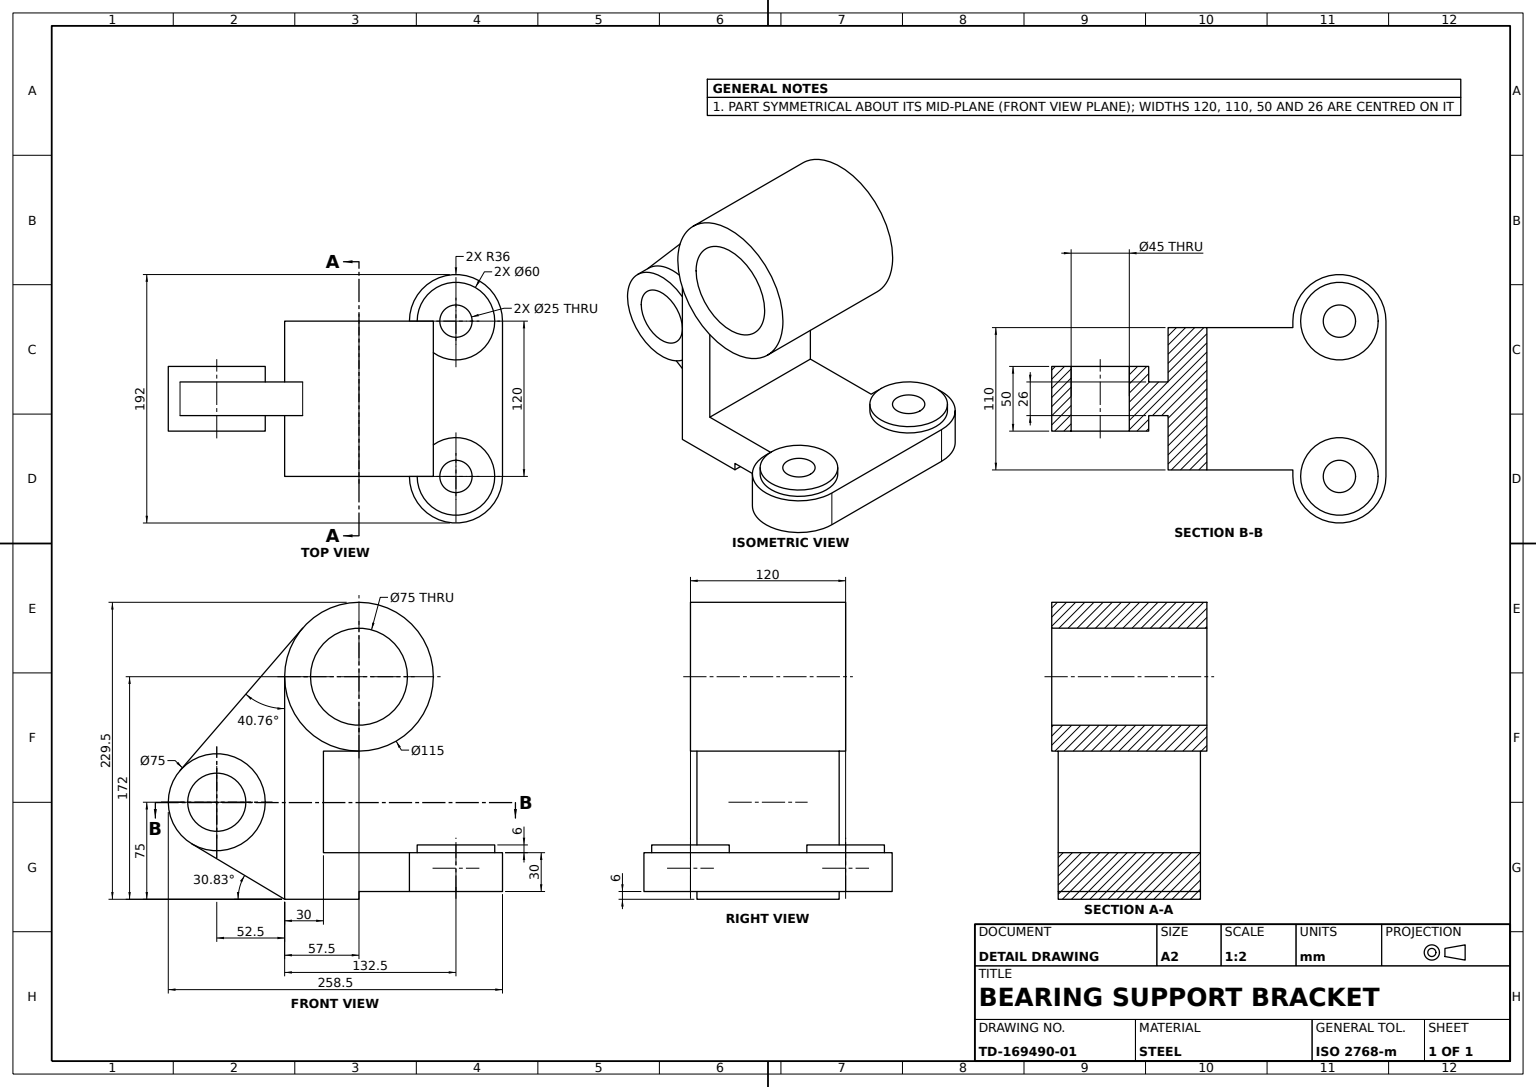
SolidWorks part; units mm, degrees
material "Plain Carbon Steel"
ref_plane "Front Plane" through (0, 0, 0) normal (0, 0, 1) x (1, 0, 0)
ref_plane "Top Plane" through (0, 0, 0) normal (0, 1, 0) x (1, 0, 0)
ref_plane "Right Plane" through (0, 0, 0) normal (1, 0, 0) x (0, 0, -1)
sketch "Bearing Housing Sketch" plane through (0, 0, 0) normal (1, 0, 0) x (0, 0, -1)
  circle A0 centre (0, 0) radius 37.5
  circle A1 centre (0, 0) radius 57.5
  dimension "D1" = 115
  dimension "D2" = 75
extrude "Bearing Housing Ø115" add sketch "Bearing Housing Sketch" against normal mid plane 120
ref_plane "Plane1" through (0, -166, 0) normal (0, 1, 0) x (1, 0, 0)
sketch "Base Foot Sketch" plane through (0, -166, 0) normal (0, 1, 0) x (1, 0, 0)
  line L0 (-60, 75) -> (60, 75) construction
  line L1 (-60, 111) -> (60, 111)
  line L2 (-60, 39) -> (60, 39)
  line L3 (-60, -57.5) -> (60, -57.5) construction
  arc A0 (-60, 111) -> (-60, 39) centre (-60, 75) ccw
  arc A1 (60, 39) -> (60, 111) centre (60, 75) ccw
  circle A2 centre (60, 75) radius 12.5
  circle A3 centre (-60, 75) radius 12.5
  point P2 (0, 75)
  dimension "D2" = 36
  dimension "D4" = 25
  dimension "D5" = 25
  dimension "D1" = 120
  dimension "D3" = 132.5
extrude "Base Foot" add sketch "Base Foot Sketch" along normal blind 30 separate body
sketch "Mounting Pad Sketch" plane through (0, -136, 0) normal (0, 1, 0) x (1, 0, 0)
  circle A0 centre (60, 75) radius 30
  circle A1 centre (-60, 75) radius 30
  circle A2 centre (60, 75) radius 12.5 construction
  circle A3 centre (-60, 75) radius 12.5 construction
  circle A4 centre (60, 75) radius 12.5
  circle A5 centre (-60, 75) radius 12.5
  dimension "D1" = 60
extrude "Mounting Pad" add sketch "Mounting Pad Sketch" along normal blind 6
sketch "Support Web Sketch" plane through (0, 0, 0) normal (1, 0, 0) x (0, 0, -1)
  line L0 (-57.5, 0) -> (-57.5, -172)
  line L1 (-57.5, -172) -> (0, -172)
  line L2 (0, -172) -> (0, -166)
  line L3 (105.6, -166) -> (-105.6, -166) construction
  line L4 (0, -166) -> (39, -166)
  line L5 (39, -136) -> (39, -166) construction
  line L6 (39, -136) -> (39, -166)
  line L7 (0, -57.5) -> (-27.5, -57.5)
  line L8 (-27.5, -57.5) -> (-27.5, -136)
  line L9 (-27.5, -136) -> (39, -136)
  circle A0 centre (0, 0) radius 57.5 construction
  arc A1 (-57.5, 0) -> (0, -57.5) centre (0, 0) ccw
  dimension "D1" = 30
  dimension "D2" = 57.5
  dimension "D3" = 6
extrude "Support Web" add sketch "Support Web Sketch" along normal mid plane 110
sketch "Side Boss Sketch" plane through (0, 0, 0) normal (1, 0, 0) x (0, 0, -1)
  line L0 (-57.5, -172) -> (0, -172) construction
  circle A0 centre (-110, -97) radius 22.5
  circle A1 centre (-110, -97) radius 37.5
  dimension "D1" = 75
  dimension "D2" = 45
  dimension "D3" = 75
  dimension "D4" = 110
extrude "Side Boss Ø75" add sketch "Side Boss Sketch" along normal mid plane 50 separate body
sketch "Gusset Rib Sketch" plane through (0, 0, 0) normal (1, 0, 0) x (0, 0, -1)
  line L0 (-138.4063, -72.5187) -> (-43.5563, 37.538)
  line L1 (-57.5, -172) -> (-129.2169, -129.2019)
  line L2 (-57.5, -172) -> (-57.5, 0)
  circle A0 centre (-110, -97) radius 37.5 construction
  circle A1 centre (0, 0) radius 57.5 construction
  arc A2 (-43.5563, 37.538) -> (-57.5, 0) centre (0, 0) ccw
  arc A3 (-129.2169, -129.2019) -> (-138.4063, -72.5187) centre (-110, -97) ccw
extrude "Gusset Rib" add sketch "Gusset Rib Sketch" along normal mid plane 26
